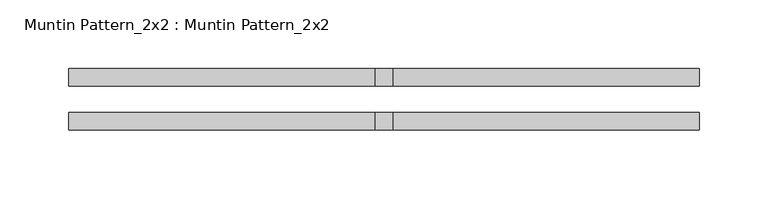
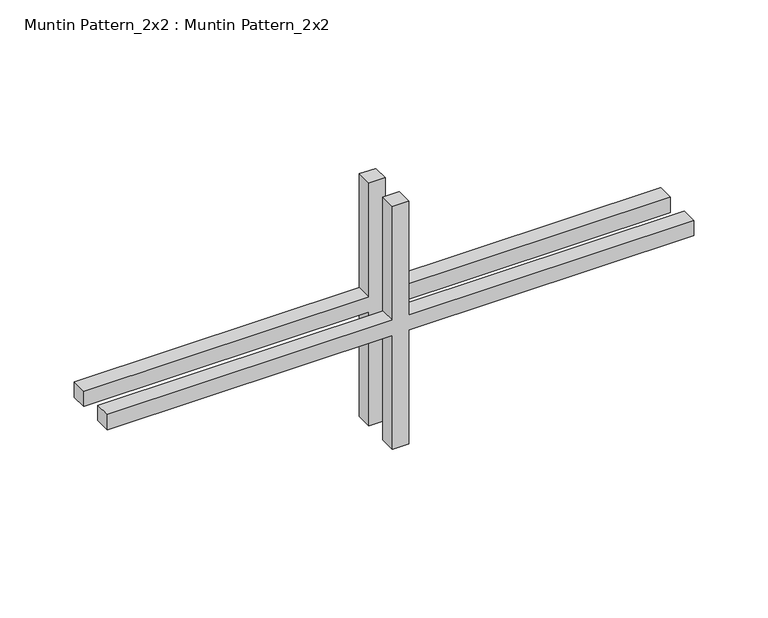
"""IFC4 building model written with IfcOpenShell, lengths in millimetres: proxy geometry, Muntin Pattern_2x2 : Muntin Pattern_2x2."""

from ifc_helpers import new_model, si_unit, frame, origin, place, context, project, spatial, polyline, outline, extrude, source, transform, mapped, element, save


def muntin_pattern_2x2_muntin_pattern_2x2_d17a704b(model_context):
    return source(origin(), model_context, "Body", "SweptSolid", [
        extrude(outline(polyline([(106.3625, -6.35), (106.3625, -228.6), (93.6625, -228.6), (93.6625, -6.35), (0.0, -6.35), (0.0, 6.35), (93.6625, 6.35), (93.6625, 228.6), (106.3625, 228.6), (106.3625, 6.35), (200.025, 6.35), (200.025, -6.35), (106.3625, -6.35)])), frame((0.0, 9.525, 0.0), z_axis=(0.0, 1.0, 0.0), x_axis=(0.0, 0.0, 1.0)), (0.0, 0.0, 1.0), 12.7),
        extrude(outline(polyline([(106.3625, -6.35), (106.3625, -228.6), (93.6625, -228.6), (93.6625, -6.35), (0.0, -6.35), (0.0, 6.35), (93.6625, 6.35), (93.6625, 228.6), (106.3625, 228.6), (106.3625, 6.35), (200.025, 6.35), (200.025, -6.35), (106.3625, -6.35)])), frame((0.0, -22.225, 0.0), z_axis=(0.0, 1.0, 0.0), x_axis=(0.0, 0.0, 1.0)), (0.0, 0.0, 1.0), 12.7),
    ])


if __name__ == "__main__":
    model = new_model("IFC4")
    model_context = context("Model", 3, world=origin())
    ifc_project = project(units=[si_unit("LENGTHUNIT", "METRE", prefix="MILLI")], contexts=[model_context])
    site = spatial("IfcSite", under=ifc_project)
    building = spatial("IfcBuilding", under=site)
    placement = place(None, origin())
    muntin_pattern_2x2_muntin_pattern_2x2_shape = muntin_pattern_2x2_muntin_pattern_2x2_d17a704b(model_context)
    element("IfcBuildingElementProxy", 1, Name="Muntin Pattern_2x2 : Muntin Pattern_2x2", ObjectType="Muntin Pattern_2x2 : Muntin Pattern_2x2", at=placement, inside=building, context=model_context, shape_type="MappedRepresentation", body=[
        mapped(muntin_pattern_2x2_muntin_pattern_2x2_shape, transform((0.0, 0.0, 0.0), x_axis=(1.0, 0.0, 0.0), y_axis=(0.0, 1.0, 0.0), z_axis=(0.0, 0.0, 1.0))),
    ])
    save(model, "model.ifc")

# Revit data of these elements
# Type "Muntin Pattern_2x2 : Muntin Pattern_2x2"
#   Width [instance default] = 4' - 0"
#   Thickness = 0' - 0 1/2"
#   Height [instance default] = 4' - 0"
#   Distance = 0' - 0 3/4"
#   Interior Material [instance default] = none
#   Exterior Material [instance default] = none
#   Default Elevation = 0
# Element 1 (IfcBuildingElementProxy, "Muntin Pattern_2x2 : Muntin Pattern_2x2")
#   Width = 1' - 6"
#   Height = 0' - 7 7/8"
#   Interior Material = Wood - Stained
#   Exterior Material = Clad - White
#   Materials on its faces: "Clad - White", "Wood - Stained"
# Materials
#   "Clad - White": class "Wood", colour RGB 242 242 238, transparency 0, Cost = 0
#   "Wood - Stained": class "Wood", colour RGB 224 178 126, transparency 0, Cost = 0
